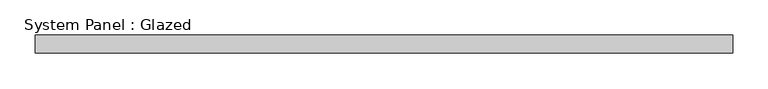
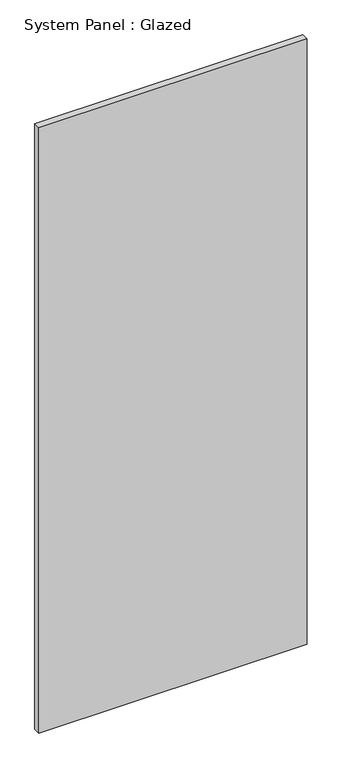
"""IFC4 building model written with IfcOpenShell, lengths in millimetres: plate geometry, System Panel : Glazed."""

from ifc_helpers import new_model, si_unit, origin, origin_with_axes, place, context, project, spatial, polyline, outline, extrude, source, transform, mapped, element, save


def system_panel_glazed_8cf484b6(model_context):
    return source(origin(), model_context, "Body", "SweptSolid", [
        extrude(outline(polyline([(491.3273704, 19.05), (-491.3273704, 19.05), (-491.3273704, 44.45), (491.3273704, 44.45), (491.3273704, 19.05)])), origin_with_axes(), (0.0, 0.0, 1.0), 2343.15),
    ])


if __name__ == "__main__":
    model = new_model("IFC4")
    model_context = context("Model", 3, world=origin())
    ifc_project = project(units=[si_unit("LENGTHUNIT", "METRE", prefix="MILLI")], contexts=[model_context])
    site = spatial("IfcSite", under=ifc_project)
    building = spatial("IfcBuilding", under=site)
    placement = place(None, origin())
    system_panel_glazed_shape = system_panel_glazed_8cf484b6(model_context)
    element("IfcPlate", 1, ObjectType="System Panel : Glazed", at=placement, inside=building, context=model_context, shape_type="MappedRepresentation", body=[
        mapped(system_panel_glazed_shape, transform((0.0, 0.0, 0.0), x_axis=(1.0, 0.0, 0.0), y_axis=(0.0, 1.0, 0.0), z_axis=(0.0, 0.0, 1.0))),
    ])
    save(model, "model.ifc")

# Revit data of these elements
# Type "System Panel : Glazed"
#   Construction Type Id = "GSP4R"
#   Analytic Construction = "1/8 in Pilkington single glazing"
#   Visual Light Transmittance = 0.9
#   Solar Heat Gain Coefficient = 0.86
#   Heat Transfer Coefficient (U) = 1.18115 BTU/(h·ft²·°F)
#   Define Thermal Properties by = 1
# Element 1 (IfcPlate, "System Panel : Glazed")
#   Materials on its faces: "Glass"
# Materials
#   "Glass": class "Glass", colour RGB 0 128 192, transparency 0.75, Description = "Soda Lime Glass", Cost = 0
